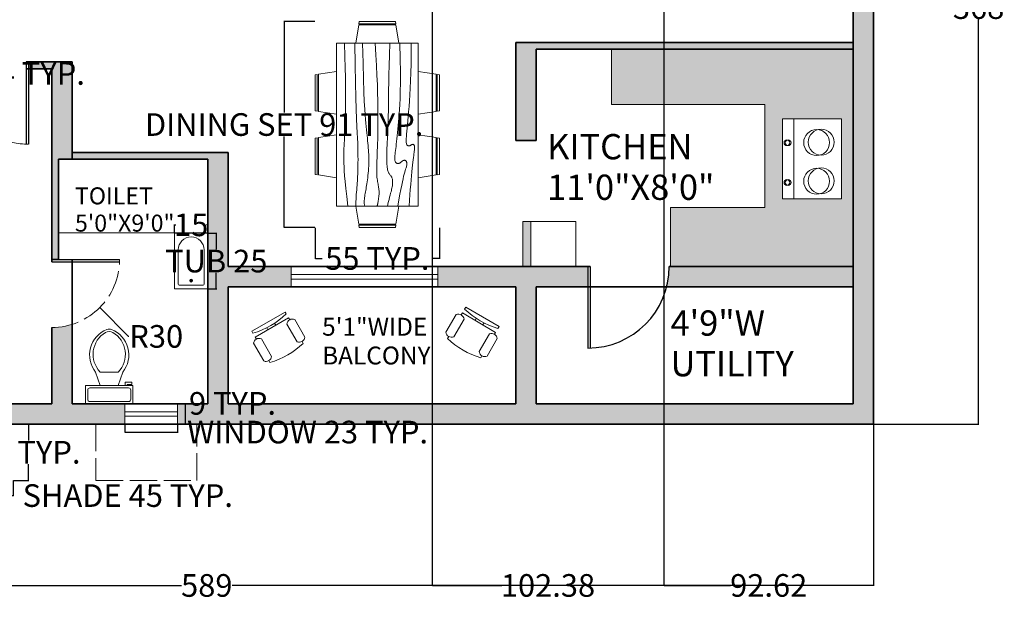
# Model space of a CAD drawing. Units: inches. Extents: x 215 to 969, y -612 to 418.
# Tile 2 of 8: x 502 to 937, y -612 to -356. Entities that reach past the tile are written whole.
import ezdxf

# ---------------------------------------------------------------- set-up
doc = ezdxf.new("R2010")
doc.units = ezdxf.units.IN
doc.header["$MEASUREMENT"] = 0
doc.linetypes.add('ACAD_ISO02W100', pattern=[15, 12, -3])
for name, color, linetype, lineweight in [('A-ANNO-DIMS', 2, 'Continuous', 18), ('A-AREA-IDEN', 7, 'Continuous', 18), ('A-DOOR', 3, 'Continuous', 25), ('A-DOOR-SWNG', 3, 'ACAD_ISO02W100', 13), ('A-EQPM', 8, 'Continuous', 18), ('A-FLOR-CASE', 9, 'Continuous', 18), ('A-FLOR-FIXT', 9, 'Continuous', 18), ('A-FLOR-OVHD', 8, 'ACAD_ISO02W100', 13), ('A-FURN', 8, 'Continuous', 18), ('A-GLAZ', 4, 'Continuous', 18), ('A-WALL', 7, 'Continuous', 35)]:
    doc.layers.add(name, color=color, linetype=linetype, lineweight=lineweight)
doc.layers.add('A-WALL-PATT', color=252, linetype='Continuous', lineweight=13, true_color=0x939598)
doc.styles.get("Standard").update_dxf_attribs({"font": 'arial.ttf'})
doc.dimstyles.get("Standard").update_dxf_attribs({"dimtxt": 10, "dimasz": 0.18, "dimexe": 0.18, "dimexo": 0.0625, "dimgap": 0.09, "dimtad": 0, "dimtih": 1, "dimtoh": 1, "dimdec": 0, "dimzin": 0, "dimdsep": 46, "dimlunit": 3, "dimtxsty": 'Standard', "dimcen": 0.09, "dimadec": 0, "dimazin": 0, "dimtfac": 1, "dimtdec": 0, "dimtofl": 0, "dimtmove": 0, "dimatfit": 3, "dimfxl": 1, "dimtolj": 1, "dimtzin": 0, "dimarcsym": 0})

# ---------------------------------------------------------------- blocks, each defined once
blk = doc.blocks.new('Dining Set - 36 x 72 in.')
for p, q in [((-22, 27.5), (-22.1562, 26.50042)), ((-5.8416, 26.5), (-22.1534, 26.5)), ((-22, 27.5), (-6, 27.5)), ((-5.8437, 26.49966), (-6, 27.5)), ((6, 27.5), (5.8438, 26.50042)), ((22.1584, 26.5), (5.8466, 26.5)), ((6, 27.5), (22, 27.5)), ((22.1563, 26.49966), (22, 27.5)), ((-22.2343, 26.00059), (-23.4847, 17.99762)), ((-22.2304, 26), (-5.7608, 26)), ((-4.5152, 17.99762), (-5.7655, 25.99926)), ((5.7657, 26.00059), (4.5153, 17.99762)), ((5.7696, 26), (22.2392, 26)), ((23.4848, 17.99762), (22.2345, 25.99926)), ((36, 18), (-36, 18)), ((-36, 18), (-36, -18)), ((36, -18), (36, 18)), ((-44.0006, 8.23428), (-35.9976, 9.48474)), ((44.0006, 8.23428), (35.9976, 9.48474)), ((-45.5, 8), (-44.5004, 8.15617)), ((-45.5, 8), (-45.5, -8)), ((-44.5, -8.15843), (-44.5, 8.15338)), ((-44, 8.23041), (-44, -8.23915)), ((44, 8.23041), (44, -8.23915)), ((44.5, -8.15843), (44.5, 8.15338)), ((45.5, 8), (44.5005, 8.15617)), ((45.5, 8), (45.5, -8)), ((-44.4997, -8.15631), (-45.5, -8)), ((-35.9976, -9.48476), (-43.9993, -8.2345)), ((35.9976, -9.48476), (43.9993, -8.2345)), ((44.4997, -8.15631), (45.5, -8)), ((-36, -18), (36, -18)), ((-22.2343, -26.0006), (-23.4847, -17.99762)), ((-4.5152, -17.99762), (-5.7655, -25.99928)), ((5.7657, -26.0006), (4.5153, -17.99762)), ((23.4848, -17.99762), (22.2345, -25.99928)), ((-22.2304, -26), (-5.7608, -26)), ((5.7696, -26), (22.2392, -26)), ((-22, -27.5), (-22.1562, -26.50044)), ((-5.8416, -26.5), (-22.1534, -26.5)), ((-22, -27.5), (-6, -27.5)), ((-5.8437, -26.49967), (-6, -27.5)), ((6, -27.5), (5.8438, -26.50044)), ((22.1584, -26.5), (5.8466, -26.5)), ((6, -27.5), (22, -27.5)), ((22.1563, -26.49967), (22, -27.5))]:
    blk.add_line(p, q)
for points in [[(-36, 15), (-31.1772, 14.97754), (-26.8079, 14.91406), (-22.8538, 14.81543), (-19.276, 14.6875), (-16.0362, 14.53613), (-13.0957, 14.36718), (-10.4159, 14.18652), (-7.9583, 14), (-5.6904, 13.81315), (-3.6035, 13.63021), (-1.6954, 13.45508), (0.0365, 13.29166), (1.5945, 13.14388), (2.9811, 13.01562), (4.1988, 12.9108), (5.25, 12.83333), (6.1393, 12.78613), (6.8802, 12.76823), (7.4883, 12.77767), (7.9792, 12.8125), (8.3685, 12.87077), (8.6719, 12.95052), (8.9049, 13.0498), (9.0833, 13.16666), (9.2205, 13.29899), (9.3216, 13.44401), (9.3895, 13.59879), (9.4271, 13.76041), (9.4373, 13.92594), (9.4232, 14.09245), (9.3875, 14.257), (9.3333, 14.41666), (9.2638, 14.56917), (9.1836, 14.71484), (9.0975, 14.85465), (9.0104, 14.98958), (8.9272, 15.1206), (8.8529, 15.2487), (8.7922, 15.37483), (8.75, 15.5), (8.7305, 15.62467), (8.7344, 15.74739), (8.7617, 15.86621), (8.8125, 15.97916), (8.8867, 16.08431), (8.9844, 16.17968), (9.1055, 16.26334), (9.25, 16.33333), (9.4189, 16.38802), (9.6172, 16.42708), (9.8506, 16.45052), (10.125, 16.45833), (10.4463, 16.45052), (10.8203, 16.42708), (11.2529, 16.38802), (11.75, 16.33333), (12.3184, 16.26318), (12.9694, 16.17838), (13.7151, 16.07991), (14.5677, 15.96875), (15.5395, 15.84586), (16.6426, 15.71224), (17.8893, 15.56884), (19.2917, 15.41666), (20.859, 15.25667), (22.5879, 15.08984), (24.4721, 14.91715), (26.5052, 14.73958), (28.6809, 14.5581), (30.9929, 14.3737), (33.4347, 14.18733), (36, 14)], [(-36, 10), (-28.9766, 10.14274), (-23.1725, 10.20442), (-18.4241, 10.19775), (-14.5677, 10.13541), (-11.4399, 10.03011), (-8.877, 9.89453), (-6.7154, 9.74137), (-4.7917, 9.58333), (-2.9698, 9.43082), (-1.2246, 9.28515), (0.4415, 9.14534), (2.026, 9.01041), (3.5266, 8.87939), (4.9408, 8.7513), (6.266, 8.62516), (7.5, 8.5), (8.6411, 8.37549), (9.6914, 8.2539), (10.6538, 8.13818), (11.5312, 8.03125), (12.3267, 7.93603), (13.043, 7.85547), (13.6831, 7.79248), (14.25, 7.75), (14.7471, 7.7303), (15.1797, 7.73307), (15.5537, 7.75732), (15.875, 7.80208), (16.1494, 7.86637), (16.3828, 7.94922), (16.5811, 8.04964), (16.75, 8.16666), (16.8944, 8.29915), (17.0143, 8.44531), (17.1089, 8.60319), (17.1771, 8.77083), (17.218, 8.94629), (17.2305, 9.1276), (17.2137, 9.31282), (17.1667, 9.5), (17.0895, 9.6875), (16.987, 9.875), (16.8649, 10.0625), (16.7292, 10.25), (16.5856, 10.4375), (16.4401, 10.625), (16.2985, 10.8125), (16.1667, 11), (16.05, 11.18733), (15.9518, 11.3737), (15.8752, 11.5581), (15.8229, 11.73958), (15.798, 11.91715), (15.8034, 12.08984), (15.842, 12.25667), (15.9167, 12.41666), (16.0295, 12.56836), (16.1784, 12.70833), (16.3605, 12.83268), (16.5729, 12.9375), (16.8127, 13.01888), (17.0768, 13.07291), (17.3625, 13.0957), (17.6667, 13.08333), (17.9894, 13.03312), (18.3418, 12.94726), (18.7382, 12.82918), (19.1927, 12.68229), (19.7195, 12.51001), (20.3327, 12.31575), (21.0465, 12.10294), (21.875, 11.875), (22.8357, 11.63354), (23.959, 11.37304), (25.2786, 11.08618), (26.8282, 10.76562), (28.6414, 10.40405), (30.752, 9.99414), (33.1936, 9.52856), (36, 9)], [(-36, 5.5), (-30.7157, 5.3348), (-26.069, 5.20963), (-21.9946, 5.11767), (-18.4271, 5.05208), (-15.3009, 5.00602), (-12.5508, 4.97265), (-10.1112, 4.94515), (-7.9167, 4.91666), (-5.909, 4.88167), (-4.0586, 4.83984), (-2.3429, 4.79215), (-0.7396, 4.73958), (0.7739, 4.6831), (2.22, 4.6237), (3.6213, 4.56233), (5, 4.5), (6.373, 4.43782), (7.7344, 4.3776), (9.0723, 4.32129), (10.375, 4.27083), (11.6309, 4.22819), (12.8281, 4.19531), (13.9551, 4.17415), (15, 4.16666), (15.954, 4.17448), (16.819, 4.19791), (17.6001, 4.23698), (18.3021, 4.29166), (18.9299, 4.36198), (19.4883, 4.44791), (19.9823, 4.54948), (20.4167, 4.66666), (20.7969, 4.79899), (21.1302, 4.94401), (21.4245, 5.09879), (21.6875, 5.26041), (21.9271, 5.42594), (22.1511, 5.59245), (22.3672, 5.757), (22.5834, 5.91666), (22.8065, 6.06868), (23.0404, 6.21093), (23.2879, 6.34147), (23.5521, 6.45833), (23.8358, 6.55957), (24.142, 6.64323), (24.4735, 6.70735), (24.8334, 6.75), (25.2235, 6.76969), (25.642, 6.76692), (26.0858, 6.74267), (26.5521, 6.69791), (27.0379, 6.63362), (27.5404, 6.55078), (28.0565, 6.45036), (28.5834, 6.33333), (29.1242, 6.19987), (29.7071, 6.04687), (30.3661, 5.87044), (31.1354, 5.66666), (32.0493, 5.43164), (33.142, 5.16146), (34.4475, 4.85221), (36, 4.5)], [(-36, -1), (-30.7915, -0.6591), (-26.0195, -0.38216), (-21.6519, -0.16284), (-17.6563, 0.00521), (-14.0005, 0.12833), (-10.6523, 0.21289), (-7.5796, 0.26522), (-4.75, 0.29166), (-2.134, 0.29793), (0.2878, 0.28711), (2.5317, 0.26163), (4.6146, 0.22396), (6.5529, 0.17651), (8.3633, 0.12174), (10.0623, 0.06209), (11.6667, 0), (13.1899, -0.06201), (14.6341, -0.1211), (15.9982, -0.17432), (17.2813, -0.21875), (18.4823, -0.25147), (19.6003, -0.26953), (20.6343, -0.27002), (21.5834, -0.25), (22.4481, -0.20768), (23.2357, -0.14584), (23.9549, -0.06836), (24.6146, 0.02083), (25.2235, 0.11784), (25.7904, 0.21875), (26.3241, 0.31966), (26.8334, 0.41666), (27.3265, 0.50618), (27.8099, 0.58593), (28.2894, 0.65397), (28.7709, 0.70833), (29.2601, 0.74707), (29.763, 0.76823), (30.2855, 0.76985), (30.8334, 0.75), (31.4088, 0.70784), (31.9994, 0.64713), (32.589, 0.57275), (33.1615, 0.48958), (33.7008, 0.4025), (34.1908, 0.3164), (34.6153, 0.23616), (34.9584, 0.16666), (35.2099, 0.11165), (35.3848, 0.07031), (35.504, 0.04069), (35.5886, 0.02083), (35.6594, 0.00879), (35.7377, 0.0026), (35.8442, 0.00032), (36, 0)], [(-36, -6.5), (-27.1843, -6.31267), (-20.084, -6.1263), (-14.469, -5.9419), (-10.1094, -5.76042), (-6.7752, -5.58285), (-4.2363, -5.41016), (-2.2629, -5.24333), (-0.625, -5.08334), (0.8708, -4.93099), (2.2715, -4.78646), (3.5872, -4.64974), (4.8281, -4.52084), (6.0046, -4.39974), (7.127, -4.28646), (8.2053, -4.18099), (9.25, -4.08334), (10.2705, -3.99382), (11.2734, -3.91407), (12.2647, -3.84603), (13.25, -3.79167), (14.2354, -3.75293), (15.2266, -3.73177), (16.2295, -3.73015), (17.25, -3.75), (18.2912, -3.79248), (19.3451, -3.85547), (20.4009, -3.93604), (21.4479, -4.03125), (22.4754, -4.13819), (23.4727, -4.25391), (24.4289, -4.37549), (25.3334, -4.5), (26.1785, -4.62492), (26.9694, -4.74935), (27.7145, -4.87281), (28.4219, -4.99479), (29.1, -5.11483), (29.7572, -5.23242), (30.4016, -5.34709), (31.0417, -5.45834), (31.6837, -5.56437), (32.3262, -5.65821), (32.9658, -5.73153), (33.599, -5.77604), (34.2224, -5.78345), (34.8327, -5.74545), (35.4264, -5.65373), (36, -5.5)], [(-36, -10), (-26.4022, -9.81299), (-18.4675, -9.62891), (-11.9839, -9.45069), (-6.7396, -9.28125), (-2.5226, -9.12354), (0.8789, -8.98047), (3.6769, -8.85498), (6.0833, -8.75), (8.2767, -8.66765), (10.3021, -8.60677), (12.1712, -8.56543), (13.8958, -8.54167), (15.4876, -8.53353), (16.9583, -8.53907), (18.3197, -8.55632), (19.5834, -8.58334), (20.7616, -8.61841), (21.8685, -8.66081), (22.9188, -8.71004), (23.9271, -8.76563), (24.9081, -8.82707), (25.8763, -8.89388), (26.8465, -8.96558), (27.8334, -9.04167), (28.8474, -9.12118), (29.8828, -9.20117), (30.93, -9.27824), (31.9792, -9.34896), (33.0205, -9.40991), (34.0443, -9.45768), (35.0407, -9.48885), (36, -9.5)], [(-36, -14.5), (-30.0881, -14.33513), (-25.0332, -14.21224), (-20.7312, -14.12647), (-17.0781, -14.07292), (-13.97, -14.04671), (-11.3027, -14.04297), (-8.9724, -14.05681), (-6.875, -14.08334), (-4.9224, -14.11833), (-3.0905, -14.16016), (-1.3709, -14.20785), (0.2448, -14.26042), (1.7647, -14.3169), (3.1973, -14.3763), (4.5507, -14.43767), (5.8333, -14.5), (7.0554, -14.5621), (8.235, -14.62175), (9.3922, -14.67652), (10.5469, -14.72396), (11.7192, -14.76164), (12.929, -14.78711), (14.1965, -14.79794), (15.5417, -14.79167), (16.9933, -14.76424), (18.6152, -14.70508), (20.4804, -14.60197), (22.6615, -14.44271), (25.2312, -14.21509), (28.2624, -13.9069), (31.8277, -13.50594), (36, -13)]]:
    blk.add_lwpolyline(points)
blk = doc.blocks.new('Bath Tub - 26 x 60 in.')
for p, q in [((8, -18), (10, -18)), ((9, -17), (9, -19))]:
    blk.add_line(p, q)
blk.add_lwpolyline([(0, -36), (0, 0), (60, 0), (60, -36)], close=True)
for points in [[(4, -30), (4, -6)], [(6, -4), (42, -4)], [(42, -32), (6, -32)]]:
    blk.add_lwpolyline(points)
for radius in [1.5, 1]:
    blk.add_circle((9, -18), radius)
for centre, radius, start, end in [((5.75, -5.75), 1.77, 81.8699, 188.1301), ((42, -18), 14, 270, 90), ((5.75, -30.25), 1.77, 171.8699, 278.1301)]:
    blk.add_arc(centre, radius, start, end)
blk = doc.blocks.new('Toilet - top')
for p, q in [((9.5, -6), (9.5, -2)), ((-10, -8.5), (-8, -8.5)), ((-10, -9.5), (-10, -8.5)), ((-8, -8.5), (-8, -8)), ((-7, -8), (-7, -9.5)), ((-4, -8), (-6, -14)), ((4, -8), (6, -14)), ((-7, -9.5), (-10, -9.5)), ((4, -14), (-4, -14))]:
    blk.add_line(p, q)
blk.add_lwpolyline([(10.5, -8), (10.5, 0), (-10.5, 0), (-10.5, -8)], close=True)
for points in [[(-9.5, -2), (-9.5, -6)], [(8.5, -1), (-8.5, -1)], [(-8.5, -7), (8.5, -7)]]:
    blk.add_lwpolyline(points)
for centre, radius, start, end in [((-8.62, -1.88), 0.884, 81.8699, 188.1301), ((8.62, -1.88), 0.884, 351.8699, 98.1301), ((-8.62, -6.12), 0.884, 171.8699, 278.1301), ((8.62, -6.12), 0.884, 261.8699, 8.1301), ((3.52, -21.58), 12.17, 141.4691, 247.9714), ((4.2, -21.82), 11.33, 136.3677, 238.9468), ((-3.52, -21.58), 12.17, 292.0284, 38.5307), ((-4.2, -21.82), 11.33, 301.053, 43.6321), ((0, -27.88), 4, 245.7318, 294.2682), ((0, -29), 4, 254.8605, 285.1395)]:
    blk.add_arc(centre, radius, start, end)
blk = doc.blocks.new('Chair - Desk')
for p, q in [((-8.5, 0), (-8.5, -1)), ((-8.5, 0), (8.5, 0)), ((8.5, 0), (8.5, -1)), ((-8.5, -3), (-8.5, -4)), ((-8.5, -3), (8.5, -3)), ((-2, -3), (-2, -1.9355)), ((2, -1.9576), (2, -3)), ((8.5, -3), (8.5, -4)), ((-10.5, -5), (-10.5, -14)), ((-6.5, -14), (-6.5, -5)), ((6.5, -5), (6.5, -14)), ((10.5, -14), (10.5, -5)), ((-8.5, -15), (-8.5, -16)), ((8.5, -15), (8.5, -16))]:
    blk.add_line(p, q)
for centre, radius, start, end in [((-8.5, -6.5), 2.5, 36.8699, 143.1301), ((0, 34.625), 36.625, 256.5803, 283.4197), ((8.5, -6.5), 2.5, 36.8699, 143.1301), ((-8.5, -12.5), 2.5, 216.8699, 323.1301), ((0, 19.625), 36.625, 256.5803, 283.4197), ((8.5, -12.5), 2.5, 216.8699, 323.1301)]:
    blk.add_arc(centre, radius, start, end)
blk = doc.blocks.new('WINDOW-SHADE-45')
for p, q in [((0, 24.86), (0, 0)), ((44.63, 0), (44.63, 24.86)), ((0, 0), (44.63, 0))]:
    blk.add_line(p, q)
blk = doc.blocks.new('DOOR-SINGLE-36')
for p, q in [((35, 0), (35, 36)), ((36, 0), (36, 36)), ((35, 0), (36, 0))]:
    blk.add_line(p, q)
blk.add_arc((36, 0), 36, 90, 180)
blk = doc.blocks.new('WIN-24')
for p, q in [((0, 9), (0, 0)), ((23.37, 9), (23.37, 0)), ((0, 5.5), (23.37, 5.5)), ((0, 3.5), (23.37, 3.5))]:
    blk.add_line(p, q)
blk = doc.blocks.new('*D33')
at = {"layer": 'A-ANNO-DIMS', "color": 0, "lineweight": -2, "transparency": 16777216}
for p, q in [((418.41, -374.51), (418.41, -379.72)), ((452.34, -374.51), (452.34, -379.72)), ((418.59, -379.54), (452.16, -379.54)), ((452.34, -379.54), (452.52, -379.54))]:
    blk.add_line(p, q, dxfattribs=at)
at = {"layer": 'A-ANNO-DIMS', "color": 0, "transparency": 16777216}
for points in [[(418.59, -379.51), (418.59, -379.57), (418.41, -379.54)], [(452.16, -379.51), (452.16, -379.57), (452.34, -379.54)]]:
    blk.add_solid(points, dxfattribs=at)
at = {"layer": 'Defpoints', "color": 0, "transparency": 16777216}
for p in [(418.41, -374.45), (452.34, -374.45), (452.34, -379.54)]:
    blk.add_point(p, dxfattribs=at)
at = {"layer": 'A-ANNO-DIMS', "color": 0, "transparency": 16777216, "insert": (492.98, -379.54), "char_height": 10, "attachment_point": 5}
blk.add_mtext('\\A1;TUB 34 TYP.', dxfattribs=at)
blk = doc.blocks.new('*D35')
at = {"layer": 'A-ANNO-DIMS', "color": 0, "lineweight": -2, "transparency": 16777216}
for p, q in [((585.42, -450.11), (589.23, -450.11)), ((589.05, -450.29), (589.05, -457.23)), ((589.05, -474.57), (589.05, -467.62)), ((585.42, -474.75), (589.23, -474.75))]:
    blk.add_line(p, q, dxfattribs=at)
at = {"layer": 'A-ANNO-DIMS', "color": 0, "transparency": 16777216}
for points in [[(589.02, -450.29), (589.08, -450.29), (589.05, -450.11)], [(589.02, -474.57), (589.08, -474.57), (589.05, -474.75)]]:
    blk.add_solid(points, dxfattribs=at)
at = {"layer": 'Defpoints', "color": 0, "transparency": 16777216}
for p in [(585.35, -450.11), (589.05, -450.11), (585.35, -474.75)]:
    blk.add_point(p, dxfattribs=at)
at = {"layer": 'A-ANNO-DIMS', "color": 0, "transparency": 16777216, "insert": (589.05, -462.43), "char_height": 10, "attachment_point": 5}
blk.add_mtext('\\A1;TUB 25', dxfattribs=at)
blk = doc.blocks.new('*D36')
at = {"layer": 'A-ANNO-DIMS', "color": 0, "lineweight": -2, "transparency": 16777216}
for p, q in [((570.57, -450.05), (570.57, -446.23)), ((570.75, -446.41), (571.14, -446.41)), ((585.17, -446.41), (584.78, -446.41)), ((585.35, -450.05), (585.35, -446.23))]:
    blk.add_line(p, q, dxfattribs=at)
at = {"layer": 'A-ANNO-DIMS', "color": 0, "transparency": 16777216}
for points in [[(570.75, -446.38), (570.75, -446.44), (570.57, -446.41)], [(585.17, -446.38), (585.17, -446.44), (585.35, -446.41)]]:
    blk.add_solid(points, dxfattribs=at)
at = {"layer": 'Defpoints', "color": 0, "transparency": 16777216}
for p in [(570.57, -446.41), (570.57, -450.11), (585.35, -450.11)]:
    blk.add_point(p, dxfattribs=at)
at = {"layer": 'A-ANNO-DIMS', "color": 0, "transparency": 16777216, "insert": (577.96, -446.41), "char_height": 10, "attachment_point": 5}
blk.add_mtext('\\A1;15', dxfattribs=at)
blk = doc.blocks.new('*D51')
at = {"layer": 'A-ANNO-DIMS', "color": 0, "lineweight": -2, "transparency": 16777216}
for p, q in [((632.61, -356.6), (618.84, -356.6)), ((619.02, -356.78), (619.02, -396.84)), ((619.02, -447.42), (619.02, -407.36)), ((632.61, -447.6), (618.84, -447.6))]:
    blk.add_line(p, q, dxfattribs=at)
at = {"layer": 'A-ANNO-DIMS', "color": 0, "transparency": 16777216}
for points in [[(618.99, -356.78), (619.05, -356.78), (619.02, -356.6)], [(618.99, -447.42), (619.05, -447.42), (619.02, -447.6)]]:
    blk.add_solid(points, dxfattribs=at)
at = {"layer": 'Defpoints', "color": 0, "transparency": 16777216}
for p in [(632.67, -356.6), (619.02, -447.6), (632.67, -447.6)]:
    blk.add_point(p, dxfattribs=at)
at = {"layer": 'A-ANNO-DIMS', "color": 0, "transparency": 16777216, "insert": (619.02, -402.1), "char_height": 10, "attachment_point": 5}
blk.add_mtext('\\A1;DINING SET 91 TYP.', dxfattribs=at)
blk = doc.blocks.new('*D52')
at = {"layer": 'A-ANNO-DIMS', "color": 0, "lineweight": -2, "transparency": 16777216}
for p, q in [((632.67, -447.67), (632.67, -461.43)), ((687.67, -447.67), (687.67, -461.43)), ((632.85, -461.25), (635.75, -461.25)), ((687.49, -461.25), (684.6, -461.25))]:
    blk.add_line(p, q, dxfattribs=at)
at = {"layer": 'A-ANNO-DIMS', "color": 0, "transparency": 16777216}
for points in [[(632.85, -461.22), (632.85, -461.28), (632.67, -461.25)], [(687.49, -461.22), (687.49, -461.28), (687.67, -461.25)]]:
    blk.add_solid(points, dxfattribs=at)
at = {"layer": 'Defpoints', "color": 0, "transparency": 16777216}
for p in [(632.67, -447.6), (687.67, -447.6), (687.67, -461.25)]:
    blk.add_point(p, dxfattribs=at)
at = {"layer": 'A-ANNO-DIMS', "color": 0, "transparency": 16777216, "insert": (660.17, -461.25), "char_height": 10, "attachment_point": 5}
blk.add_mtext('\\A1;55 TYP.', dxfattribs=at)
blk = doc.blocks.new('*D61')
at = {"layer": 'A-ANNO-DIMS', "color": 0, "lineweight": -2, "transparency": 16777216}
for p, q in [((454.72, -559.38), (454.72, -566.19)), ((499.35, -559.38), (499.35, -566.19)), ((454.9, -566.01), (499.17, -566.01)), ((499.35, -566.01), (499.53, -566.01))]:
    blk.add_line(p, q, dxfattribs=at)
at = {"layer": 'A-ANNO-DIMS', "color": 0, "transparency": 16777216}
for points in [[(454.9, -565.98), (454.9, -566.04), (454.72, -566.01)], [(499.17, -565.98), (499.17, -566.04), (499.35, -566.01)]]:
    blk.add_solid(points, dxfattribs=at)
at = {"layer": 'Defpoints', "color": 0, "transparency": 16777216}
for p in [(454.72, -559.31), (499.35, -559.31), (499.35, -566.01)]:
    blk.add_point(p, dxfattribs=at)
at = {"layer": 'A-ANNO-DIMS', "color": 0, "transparency": 16777216, "insert": (549.94, -566.01), "char_height": 10, "attachment_point": 5}
blk.add_mtext('\\A1;SHADE 45 TYP.', dxfattribs=at)
blk = doc.blocks.new('*D62')
at = {"layer": 'A-ANNO-DIMS', "color": 0, "lineweight": -2, "transparency": 16777216}
for p, q in [((499.42, -534.45), (506.23, -534.45)), ((506.05, -534.63), (506.05, -541.69)), ((506.05, -559.13), (506.05, -552.08)), ((499.42, -559.31), (506.23, -559.31))]:
    blk.add_line(p, q, dxfattribs=at)
at = {"layer": 'A-ANNO-DIMS', "color": 0, "transparency": 16777216}
for points in [[(506.02, -534.63), (506.08, -534.63), (506.05, -534.45)], [(506.02, -559.13), (506.08, -559.13), (506.05, -559.31)]]:
    blk.add_solid(points, dxfattribs=at)
at = {"layer": 'Defpoints', "color": 0, "transparency": 16777216}
for p in [(499.35, -534.45), (506.05, -534.45), (499.35, -559.31)]:
    blk.add_point(p, dxfattribs=at)
at = {"layer": 'A-ANNO-DIMS', "color": 0, "transparency": 16777216, "insert": (506.05, -546.88), "char_height": 10, "attachment_point": 5}
blk.add_mtext('\\A1;25 TYP.', dxfattribs=at)
blk = doc.blocks.new('*D65')
at = {"layer": 'A-ANNO-DIMS', "color": 0, "lineweight": -2, "transparency": 16777216}
for p, q in [((548.6, -534.51), (548.6, -538.14)), ((571.97, -534.51), (571.97, -538.14)), ((548.78, -537.96), (571.79, -537.96)), ((571.97, -537.96), (572.15, -537.96))]:
    blk.add_line(p, q, dxfattribs=at)
at = {"layer": 'A-ANNO-DIMS', "color": 0, "transparency": 16777216}
for points in [[(548.78, -537.93), (548.78, -537.99), (548.6, -537.96)], [(571.79, -537.93), (571.79, -537.99), (571.97, -537.96)]]:
    blk.add_solid(points, dxfattribs=at)
at = {"layer": 'Defpoints', "color": 0, "transparency": 16777216}
for p in [(548.6, -534.45), (571.97, -534.45), (571.97, -537.96)]:
    blk.add_point(p, dxfattribs=at)
at = {"layer": 'A-ANNO-DIMS', "color": 0, "transparency": 16777216, "insert": (629.37, -537.96), "char_height": 10, "attachment_point": 5}
blk.add_mtext('\\A1;WINDOW 23 TYP.', dxfattribs=at)
blk = doc.blocks.new('*D66')
at = {"layer": 'A-ANNO-DIMS', "color": 0, "lineweight": -2, "transparency": 16777216}
for p, q in [((572.03, -525.45), (575.65, -525.45)), ((575.47, -525.45), (575.47, -525.27)), ((575.47, -525.27), (575.65, -525.27)), ((575.47, -534.27), (575.47, -525.63)), ((572.03, -534.45), (575.65, -534.45))]:
    blk.add_line(p, q, dxfattribs=at)
at = {"layer": 'A-ANNO-DIMS', "color": 0, "transparency": 16777216}
for points in [[(575.44, -525.63), (575.5, -525.63), (575.47, -525.45)], [(575.44, -534.27), (575.5, -534.27), (575.47, -534.45)]]:
    blk.add_solid(points, dxfattribs=at)
at = {"layer": 'Defpoints', "color": 0, "transparency": 16777216}
for p in [(571.97, -525.45), (575.47, -525.45), (571.97, -534.45)]:
    blk.add_point(p, dxfattribs=at)
at = {"layer": 'A-ANNO-DIMS', "color": 0, "transparency": 16777216, "insert": (596.2, -525.27), "char_height": 10, "attachment_point": 5}
blk.add_mtext('\\A1;9 TYP.', dxfattribs=at)
blk = doc.blocks.new('*D72')
at = {"layer": 'A-ANNO-DIMS', "color": 0, "lineweight": -2, "transparency": 16777216}
for p, q in [((879.42, -166.45), (925.93, -166.45)), ((925.75, -166.63), (925.75, -345.25)), ((925.75, -534.27), (925.75, -355.65)), ((879.42, -534.45), (925.93, -534.45))]:
    blk.add_line(p, q, dxfattribs=at)
at = {"layer": 'A-ANNO-DIMS', "color": 0, "transparency": 16777216}
for points in [[(925.72, -166.63), (925.78, -166.63), (925.75, -166.45)], [(925.72, -534.27), (925.78, -534.27), (925.75, -534.45)]]:
    blk.add_solid(points, dxfattribs=at)
at = {"layer": 'Defpoints', "color": 0, "transparency": 16777216}
for p in [(879.35, -166.45), (879.35, -534.45), (925.75, -534.45)]:
    blk.add_point(p, dxfattribs=at)
at = {"layer": 'A-ANNO-DIMS', "color": 0, "transparency": 16777216, "insert": (925.75, -350.45), "char_height": 10, "attachment_point": 5}
blk.add_mtext('\\A1;368', dxfattribs=at)
blk = doc.blocks.new('*D75')
at = {"layer": 'A-ANNO-DIMS', "color": 0, "lineweight": -2, "transparency": 16777216}
for p, q in [((290.35, 103.15), (290.35, -605.89)), ((879.35, -534.51), (879.35, -605.89)), ((290.53, -605.71), (573.71, -605.71)), ((879.17, -605.71), (596, -605.71))]:
    blk.add_line(p, q, dxfattribs=at)
at = {"layer": 'A-ANNO-DIMS', "color": 0, "transparency": 16777216}
for points in [[(290.53, -605.68), (290.53, -605.74), (290.35, -605.71)], [(879.17, -605.68), (879.17, -605.74), (879.35, -605.71)]]:
    blk.add_solid(points, dxfattribs=at)
at = {"layer": 'Defpoints', "color": 0, "transparency": 16777216}
for p in [(290.35, 103.21), (879.35, -534.45), (879.35, -605.71)]:
    blk.add_point(p, dxfattribs=at)
at = {"layer": 'A-ANNO-DIMS', "color": 0, "transparency": 16777216, "insert": (584.85, -605.71), "char_height": 10, "attachment_point": 5}
blk.add_mtext('\\A1;589', dxfattribs=at)
blk = doc.blocks.new('*D76')
at = {"layer": 'A-ANNO-DIMS', "color": 0, "lineweight": -2, "transparency": 16777216}
for p, q in [((569.29, 365.5), (243.77, 365.5)), ((243.95, 365.32), (243.95, -91.71)), ((243.95, -559.13), (243.95, -102.1)), ((454.66, -559.31), (243.77, -559.31))]:
    blk.add_line(p, q, dxfattribs=at)
at = {"layer": 'A-ANNO-DIMS', "color": 0, "transparency": 16777216}
for points in [[(243.92, 365.32), (243.98, 365.32), (243.95, 365.5)], [(243.92, -559.13), (243.98, -559.13), (243.95, -559.31)]]:
    blk.add_solid(points, dxfattribs=at)
at = {"layer": 'Defpoints', "color": 0, "transparency": 16777216}
for p in [(569.35, 365.5), (243.95, -559.31), (454.72, -559.31)]:
    blk.add_point(p, dxfattribs=at)
at = {"layer": 'A-ANNO-DIMS', "color": 0, "transparency": 16777216, "insert": (243.95, -96.91), "char_height": 10, "attachment_point": 5}
blk.add_mtext('\\A1;924.8', dxfattribs=at)
blk = doc.blocks.new('*D79')
at = {"layer": 'A-ANNO-DIMS', "color": 0, "lineweight": -2, "transparency": 16777216}
for p, q in [((684.35, -82.85), (684.35, -605.89)), ((786.74, -82.85), (786.74, -605.89)), ((684.53, -605.71), (715.16, -605.71)), ((786.56, -605.71), (755.93, -605.71))]:
    blk.add_line(p, q, dxfattribs=at)
at = {"layer": 'A-ANNO-DIMS', "color": 0, "transparency": 16777216}
for points in [[(684.53, -605.68), (684.53, -605.74), (684.35, -605.71)], [(786.56, -605.68), (786.56, -605.74), (786.74, -605.71)]]:
    blk.add_solid(points, dxfattribs=at)
at = {"layer": 'Defpoints', "color": 0, "transparency": 16777216}
for p in [(684.35, -82.79), (786.74, -82.79), (786.74, -605.71)]:
    blk.add_point(p, dxfattribs=at)
at = {"layer": 'A-ANNO-DIMS', "color": 0, "transparency": 16777216, "insert": (735.55, -605.71), "char_height": 10, "attachment_point": 5}
blk.add_mtext('\\A1;102.38', dxfattribs=at)
blk = doc.blocks.new('*D81')
at = {"layer": 'A-ANNO-DIMS', "color": 0, "lineweight": -2, "transparency": 16777216}
for p, q in [((786.74, -46.85), (786.74, -605.89)), ((879.35, -46.85), (879.35, -605.89)), ((786.92, -605.71), (816.13, -605.71)), ((879.17, -605.71), (849.96, -605.71))]:
    blk.add_line(p, q, dxfattribs=at)
at = {"layer": 'A-ANNO-DIMS', "color": 0, "transparency": 16777216}
for points in [[(786.92, -605.68), (786.92, -605.74), (786.74, -605.71)], [(879.17, -605.68), (879.17, -605.74), (879.35, -605.71)]]:
    blk.add_solid(points, dxfattribs=at)
at = {"layer": 'Defpoints', "color": 0, "transparency": 16777216}
for p in [(786.74, -46.79), (879.35, -46.79), (879.35, -605.71)]:
    blk.add_point(p, dxfattribs=at)
at = {"layer": 'A-ANNO-DIMS', "color": 0, "transparency": 16777216, "insert": (833.05, -605.71), "char_height": 10, "attachment_point": 5}
blk.add_mtext('\\A1;92.62', dxfattribs=at)
blk = doc.blocks.new('*D87')
at = {"layer": 'A-ANNO-DIMS', "color": 0, "lineweight": -2, "transparency": 16777216}
for p, q in [((516.26, -461.75), (516.44, -461.75)), ((516.35, -461.84), (516.35, -461.66)), ((550.29, -495.69), (537.69, -483.09)), ((550.47, -495.69), (550.29, -495.69))]:
    blk.add_line(p, q, dxfattribs=at)
at = {"layer": 'A-ANNO-DIMS', "color": 0, "transparency": 16777216}
blk.add_solid([(537.72, -483.06), (537.67, -483.11), (537.57, -482.96)], dxfattribs=at)
at = {"layer": 'Defpoints', "color": 0, "transparency": 16777216}
for p in [(516.35, -461.75), (537.57, -482.96)]:
    blk.add_point(p, dxfattribs=at)
at = {"layer": 'A-ANNO-DIMS', "color": 0, "transparency": 16777216, "insert": (562.5, -495.69), "char_height": 10, "attachment_point": 5}
blk.add_mtext('\\A1;R30', dxfattribs=at)

msp = doc.modelspace()

# ---------------------------------------------------------------- hatches: boundary and pattern name
at = {"layer": 'A-WALL-PATT'}
h = msp.add_hatch(color=256, dxfattribs=at)
h.dxf.hatch_style = 1
h.paths.add_polyline_path([(723.3535, -175.4525), (714.3535, -175.4525), (714.3535, -205.9065), (720.3535, -205.9065), (720.3535, -314.4525), (723.3535, -314.4525)])
h.paths.add_polyline_path([(720.3535, -311.4525), (714.3535, -311.4525), (714.3535, -314.4525), (720.3535, -314.4525)], flags=17)
h.paths.add_polyline_path([(879.3535, -228.5449, -0.06325422), (870.3535, -227.4017), (870.3535, -314.4525), (870.3535, -410.4525), (870.3535, -464.8456), (870.3535, -525.4525), (730.3535, -525.4525), (730.3535, -473.8456), (753.1403, -473.8456), (753.1403, -464.8456), (686.9324, -464.8456), (686.9324, -473.8456), (721.3535, -473.8456), (721.3535, -525.4525), (594.3535, -525.4525), (594.3535, -473.8456), (622.1543, -473.8456), (622.1543, -464.8456), (594.3535, -464.8456), (594.3535, -414.4525), (525.3535, -414.4525), (525.3535, -417.4525), (585.3535, -417.4525), (585.3535, -525.4525), (571.9682, -525.4525), (571.9682, -534.4525), (879.3535, -534.4525), (879.3535, -410.4525), (879.3535, -314.4525)])
h.paths.add_polyline_path([(730.3535, -368.8456), (870.3535, -368.8456), (870.3535, -365.8456), (721.3535, -365.8456), (721.3535, -368.8456), (721.3535, -409.1143), (730.3535, -409.1143)], flags=17)
h.paths.add_polyline_path([(870.3535, -410.4525), (870.3535, -368.8456), (763.5487, -368.8456), (763.5487, -393.1792), (831.3894, -393.1792), (831.3894, -438.7284), (789.7386, -438.7284), (789.7386, -464.8456), (870.3535, -464.8456)], flags=17)
h.paths.add_polyline_path([(839.0857, -434.8848), (839.0857, -399.5193), (865.1757, -399.5193), (865.1757, -434.8848)], flags=16)
h.paths.add_polyline_path([(839.8092, -427.6923, -0.48074962), (841.3551, -426.456, -0.48074962), (842.901, -427.6923, -0.48074962), (841.3551, -428.9285, -0.48074962)], flags=0)
h.paths.add_polyline_path([(848.5001, -427.1588, -0.44021274), (854.7228, -421.4606, -0.49540019), (861.9637, -426.9752, -0.44021274), (855.741, -432.6734, -0.49540019)], flags=0)
h.paths.add_polyline_path([(848.5001, -410.0762, -0.44021274), (854.7228, -404.378, -0.49540019), (861.9637, -409.8925, -0.44021274), (855.741, -415.5907, -0.49540019)], flags=0)
h.paths.add_polyline_path([(839.8092, -410.149, -0.48074962), (841.3551, -408.9127, -0.48074962), (842.901, -410.149, -0.48074962), (841.3551, -411.3852, -0.48074962)], flags=0)
h.paths.add_polyline_path([(870.3535, -464.8456), (789.7386, -464.8456), (789.1403, -464.8456, -0.06325422), (787.9971, -473.8456), (870.3535, -473.8456)], flags=17)
h.paths.add_polyline_path([(727.9401, -444.9303), (724.3796, -444.9303), (724.3796, -464.8456), (727.9401, -464.8456)], flags=17)
h.paths.add_polyline_path([(548.597, -525.4525), (531.2503, -525.4525), (525.3535, -525.4525), (525.3535, -490.3641, -0.07632083), (516.3535, -491.7459), (516.3535, -525.4525), (488.9462, -525.4525), (488.9462, -534.4525), (548.597, -534.4525)])
h.paths.add_polyline_path([(525.3535, -374.4525), (506.0702, -374.4525), (506.0702, -377.4525), (516.3535, -377.4525), (516.3535, -461.7459), (519.3535, -461.7459), (519.3535, -417.4525), (525.3535, -417.4525), (525.3535, -414.4525)])
h.paths.add_polyline_path([(470.1724, -377.4525), (449.6899, -377.4525), (344.3535, -377.4525), (344.3535, -400.7118), (335.3535, -400.7118), (335.3535, -355.0472), (344.3535, -355.0472), (344.3535, -374.4525), (373.6368, -374.4525), (373.6368, -366.4525), (380.1368, -366.4525), (378.1369, -360.4526, -0.50132349), (383.0921, -341.5914, -0.13289091), (385.1815, -341.5914, -0.50131678), (390.1369, -360.4524), (388.1368, -366.4525), (391.1368, -366.4525), (391.1368, -364.9525), (394.1368, -364.9525), (394.1368, -365.9525), (392.1368, -365.9525), (392.1368, -366.4525), (394.6368, -366.4525), (394.6368, -374.4525), (418.4066, -374.4525), (418.4066, -354.0926), (452.3535, -354.0926), (452.3535, -374.4525), (470.0713, -374.4525, 0.02085422)])
h.paths.add_polyline_path([(442.1598, -372.1903), (421.7999, -372.1903, -0.50000012), (420.6688, -371.0592), (420.6688, -357.4859, -0.50000012), (421.7999, -356.3548), (442.1598, -356.3548, -1)], flags=16)
h.paths.add_polyline_path([(422.6483, -364.2725, -1), (424.3449, -364.2725, -1)], flags=0)
h.paths.add_polyline_path([(422.931, -364.2725, -1), (424.0621, -364.2725, -1)], flags=0)
h.paths.add_polyline_path([(392.6368, -373.4525), (375.6368, -373.4525, -0.50000012), (374.6368, -372.4525), (374.6368, -368.4525, -0.50000012), (375.6368, -367.4525), (392.6368, -367.4525, -0.50000012), (393.6368, -368.4525), (393.6368, -372.4525, -0.50000012)], flags=16)
h.paths.add_polyline_path([(388.1368, -360.4525), (380.1368, -360.4525, -0.4800795), (382.4928, -342.9295, -0.21500378), (385.7809, -342.9295, -0.48007965)], flags=16)
h.paths.add_polyline_path([(344.3535, -437.1356), (335.3535, -437.1356), (335.3535, -525.4525), (335.3535, -534.4525), (465.575, -534.4525), (465.575, -525.4525), (344.3535, -525.4525)])
h.paths.add_polyline_path([(342.2824, -347.0067), (391.5718, -347.0067), (391.5718, -334.5799), (342.2824, -334.5799)], flags=9)

# ---------------------------------------------------------------- linework, layer by layer
at = {"layer": 'A-DOOR'}
for p, q in [((505.0702, -374.4525), (505.0702, -410.7412)), ((506.0702, -374.4525), (506.0702, -410.7412)), ((519.3535, -461.7459), (516.3535, -461.7459)), ((516.3535, -461.7459), (546.3535, -461.7459)), ((516.3535, -461.7459), (516.3535, -462.7459)), ((516.3535, -462.7459), (546.3535, -462.7459)), ((753.1403, -464.8456), (753.1403, -473.8456))]:
    msp.add_line(p, q, dxfattribs=at)
at = {"layer": 'A-DOOR-SWNG'}
for centre, radius, start, end in [((506.0702, -374.7412), 36, 179.540554, 270), ((516.3535, -461.7459), 30, 270, 0)]:
    msp.add_arc(centre, radius, start, end, dxfattribs=at)
at = {"layer": 'A-EQPM'}
msp.add_line((844.1057, -399.5193), (844.1057, -434.8848), dxfattribs=at)
msp.add_lwpolyline([(839.0857, -399.5193), (865.1757, -399.5193), (865.1757, -434.8848), (839.0857, -434.8848)], close=True, dxfattribs=at)
for centre, radius in [((854.2204, -410.0762), 5.7203), ((856.2434, -409.8925), 5.7203), ((841.0764, -410.149), 1.2672), ((841.6338, -410.149), 1.2672), ((854.2204, -427.1588), 5.7203), ((856.2434, -426.9752), 5.7203), ((841.0764, -427.6923), 1.2672), ((841.6338, -427.6923), 1.2672)]:
    msp.add_circle(centre, radius, dxfattribs=at)
at = {"layer": 'A-FLOR-CASE'}
for p, q in [((763.5487, -368.8456), (763.5487, -393.1792)), ((763.5487, -393.1792), (831.3894, -393.1792)), ((831.3894, -393.1792), (831.3894, -438.7284)), ((831.3894, -438.7284), (789.7386, -438.7284)), ((789.7386, -438.7284), (789.7386, -464.8456)), ((724.3796, -464.8456), (724.3796, -444.9303)), ((724.3796, -444.9303), (727.9401, -444.9303)), ((727.9401, -444.9303), (727.9401, -464.8456)), ((727.9401, -444.9303), (747.835, -444.9303)), ((747.835, -444.9303), (747.835, -464.8456))]:
    msp.add_line(p, q, dxfattribs=at)
at = {"layer": 'A-FLOR-FIXT'}
msp.add_line((519.3535, -449.9525), (585.3535, -449.9525), dxfattribs=at)
at = {"layer": 'A-GLAZ'}
for p, q in [((622.1543, -473.8456), (622.1543, -464.8456)), ((686.9324, -464.8456), (686.9324, -473.8456)), ((622.1543, -468.3456), (686.9324, -468.3456)), ((622.1543, -470.3456), (686.9324, -470.3456))]:
    msp.add_line(p, q, dxfattribs=at)
at = {"layer": 'A-WALL'}
for p, q in [((870.3535, -314.4525), (870.3535, -410.4525)), ((879.3535, -314.4525), (879.3535, -410.4525)), ((721.3535, -368.8456), (721.3535, -365.8456)), ((721.3535, -365.8456), (870.3535, -365.8456)), ((721.3535, -409.1143), (721.3535, -368.8456)), ((870.3535, -368.8456), (730.3535, -368.8456)), ((730.3535, -368.8456), (730.3535, -409.1143)), ((870.3535, -464.8456), (870.3535, -368.8456)), ((525.3535, -374.4525), (505.0702, -374.4525)), ((516.3535, -377.4525), (505.0702, -377.4525)), ((516.3535, -462.7459), (516.3535, -377.4525)), ((525.3535, -417.4525), (525.3535, -374.4525)), ((730.3535, -409.1143), (721.3535, -409.1143)), ((879.3535, -410.4525), (879.3535, -534.4525)), ((519.3535, -417.4525), (519.3535, -461.7459)), ((519.3535, -417.4525), (525.3535, -417.4525)), ((594.3535, -414.4525), (525.3535, -414.4525)), ((585.3535, -417.4525), (525.3535, -417.4525)), ((585.3535, -525.4525), (585.3535, -417.4525)), ((594.3535, -464.8456), (594.3535, -414.4525)), ((870.3535, -414.4525), (870.3535, -525.4525)), ((879.3535, -414.4525), (879.3535, -525.4525)), ((525.3535, -525.4525), (525.3535, -461.7459)), ((594.3535, -464.8456), (721.3535, -464.8456)), ((594.3535, -464.8456), (754.1403, -464.8456)), ((789.1403, -464.8456), (870.3535, -464.8456)), ((594.3535, -525.4525), (594.3535, -473.8456)), ((594.3535, -525.4525), (594.3535, -473.8456)), ((594.3535, -473.8456), (721.3535, -473.8456)), ((721.3535, -525.4525), (721.3535, -473.8456)), ((730.3535, -525.4525), (730.3535, -473.8456)), ((730.3535, -473.8456), (870.3535, -473.8456)), ((516.3535, -525.4525), (516.3535, -491.7459)), ((344.3535, -525.4525), (516.3535, -525.4525)), ((525.3535, -525.4525), (585.3535, -525.4525)), ((594.3535, -525.4525), (721.3535, -525.4525)), ((870.3535, -525.4525), (730.3535, -525.4525)), ((879.3535, -534.4525), (335.3535, -534.4525)), ((344.3535, -534.4525), (516.3535, -534.4525)), ((525.3535, -534.4525), (585.3535, -534.4525)), ((594.3535, -534.4525), (721.3535, -534.4525)), ((870.3535, -534.4525), (730.3535, -534.4525))]:
    msp.add_line(p, q, dxfattribs=at)

# ---------------------------------------------------------------- block references
at = {"layer": 'A-DOOR', "rotation": 180}
msp.add_blockref('DOOR-SINGLE-36', (789.1408, -464.846), dxfattribs=at)
at = {"layer": 'A-FLOR-FIXT', "xscale": 0.4106632175604876, "yscale": 0.4106632175604876, "zscale": 0.4106632175604876, "rotation": 90}
msp.add_blockref('Bath Tub - 26 x 60 in.', (570.5696, -474.7486), dxfattribs=at)
at = {"layer": 'A-FLOR-FIXT', "rotation": 180}
msp.add_blockref('Toilet - top', (541.7503, -525.4525), dxfattribs=at)
at = {"layer": 'A-FLOR-OVHD'}
msp.add_blockref('WINDOW-SHADE-45', (535.8697, -559.313), dxfattribs=at)
at = {"layer": 'A-FURN'}
for name, p, rotation in [('Dining Set - 36 x 72 in.', (660.1748, -402.1035), 270), ('Chair - Desk', (706.6005, -487.0319), 329.8016705482103), ('Chair - Desk', (612.1018, -489.1662), 30.00000000000134)]:
    msp.add_blockref(name, p, dxfattribs=dict(at, rotation=rotation))
at = {"layer": 'A-GLAZ'}
msp.add_blockref('WIN-24', (548.597, -534.452), dxfattribs=at)

# ---------------------------------------------------------------- texts
at = {"layer": 'A-AREA-IDEN'}
for s, height, p in [('KITCHEN', 11.16071, (735.1678, -417.4529)), ('11\'0"X8\'0"', 11.16071, (735.1678, -435.3816)), ('TOILET ', 7.49941, (526.6197, -437.351)), ('5\'0"X9\'0"', 7.49941, (526.6197, -449.3981)), ('5\'1"WIDE', 7.90467, (635.7947, -495.3804)), ('4\'9"W', 11.16071, (789.6612, -495.3804)), ('BALCONY', 7.90467, (635.7947, -508.0785)), ('UTILITY', 11.16071, (789.6612, -513.3091))]:
    msp.add_text(s, height=height, dxfattribs=at).set_placement(p)

# ---------------------------------------------------------------- dimensions: what is measured, and where the dimension line sits
at = {"layer": 'A-ANNO-DIMS'}
for base, p1, p2, angle, override, picture, middle in [((243.9535, -559.3132), (569.3535, 365.5008), (454.7218, -559.3132), 90, {"dimdec": 1, "dimlfac": 1, "dimrnd": 0, "dimzin": 0, "dimdsep": 46, "dimlunit": 2}, '*D76', (243.9535, -96.9062)), ((925.7535, -534.4525), (879.3535, -166.4525), (879.3535, -534.4525), 90, {"dimdec": 0, "dimlfac": 1, "dimrnd": 0, "dimzin": 0, "dimdsep": 46, "dimlunit": 2}, '*D72', (925.7535, -350.4525)), ((570.5696, -446.4128), (585.3535, -450.1088), (570.5696, -450.1088), 180, {"dimdec": 0, "dimlfac": 1, "dimrnd": 0, "dimzin": 0, "dimdsep": 46, "dimlunit": 2}, '*D36', (577.9616, -446.4128))]:
    dim = msp.add_linear_dim(base=base, p1=p1, p2=p2, angle=angle, dimstyle='Standard', override=override, dxfattribs=at)
    dim.commit()
    dim.dimension.update_dxf_attribs({"geometry": picture, "text_midpoint": middle})
for base, p1, p2, override, picture, middle in [((879.3535, -605.7132), (290.3535, 103.2135), (879.3535, -534.4525), {"dimdec": 0, "dimlfac": 1, "dimrnd": 0, "dimzin": 0, "dimdsep": 46, "dimlunit": 2}, '*D75', (584.8535, -605.7132)), ((879.35349, -605.71316), (786.73847, -46.78645), (879.35349, -46.78645), {"dimdec": 2, "dimlfac": 1, "dimrnd": 0, "dimzin": 0, "dimdsep": 46, "dimlunit": 2}, '*D81', (833.04598, -605.71316)), ((786.73847, -605.71316), (684.35349, -82.78645), (786.73847, -82.78645), {"dimdec": 2, "dimlfac": 1, "dimrnd": 0, "dimzin": 0, "dimdsep": 46, "dimlunit": 2}, '*D79', (735.54598, -605.71316))]:
    dim = msp.add_linear_dim(base=base, p1=p1, p2=p2, dimstyle='Standard', override=override, dxfattribs=at)
    dim.commit()
    dim.dimension.update_dxf_attribs({"geometry": picture, "text_midpoint": middle})
for base, p1, p2, text, picture, middle in [((452.3398, -379.5425), (418.4066, -374.4525), (452.3398, -374.4525), 'TUB <> TYP.', '*D33', (492.9849, -379.5425)), ((687.6748, -461.2535), (632.6748, -447.6035), (687.6748, -447.6035), '<> TYP.', '*D52', (660.1748, -461.2535)), ((571.9682, -537.9582), (548.597, -534.4525), (571.9682, -534.4525), 'WINDOW <> TYP.', '*D65', (629.3698, -537.9582)), ((499.3531, -566.0078), (454.7218, -559.3132), (499.3531, -559.3132), 'SHADE <> TYP.', '*D61', (549.9437, -566.0078))]:
    dim = msp.add_linear_dim(base=base, p1=p1, p2=p2, text=text, dimstyle='Standard', override={"dimdec": 0, "dimlfac": 1, "dimrnd": 0, "dimzin": 0, "dimdsep": 46, "dimlunit": 2}, dxfattribs=at)
    dim.commit()
    dim.dimension.update_dxf_attribs({"geometry": picture, "text_midpoint": middle})
for base, p1, p2, angle, text, picture, middle in [((619.0248, -447.6035), (632.6748, -356.6035), (632.6748, -447.6035), 270, 'DINING SET <> TYP.', '*D51', (619.0248, -402.1035)), ((589.0495, -450.1088), (585.3535, -474.7486), (585.3535, -450.1088), 90, 'TUB <>', '*D35', (589.0495, -462.4287)), ((575.4739, -525.4525), (571.9682, -534.4525), (571.9682, -525.4525), 90, '<> TYP.', '*D66', (596.1975, -525.2725)), ((506.0478, -534.4525), (499.3531, -559.3132), (499.3531, -534.4525), 90, '<> TYP.', '*D62', (506.0478, -546.8828))]:
    dim = msp.add_linear_dim(base=base, p1=p1, p2=p2, angle=angle, text=text, dimstyle='Standard', override={"dimdec": 0, "dimlfac": 1, "dimrnd": 0, "dimzin": 0, "dimdsep": 46, "dimlunit": 2}, dxfattribs=at)
    dim.commit()
    dim.dimension.update_dxf_attribs({"geometry": picture, "text_midpoint": middle})
dim = msp.add_radius_dim(center=(516.3535, -461.7459), mpoint=(537.5669, -482.9589), dimstyle='Standard', override={"dimdec": 0, "dimlfac": 1, "dimrnd": 0, "dimzin": 0, "dimdsep": 46, "dimlunit": 2}, dxfattribs=at)
dim.commit()
dim.dimension.update_dxf_attribs({"geometry": '*D87', "text_midpoint": (562.4954, -495.6867), "dimtype": 164})

doc.saveas('drawing.dxf')
